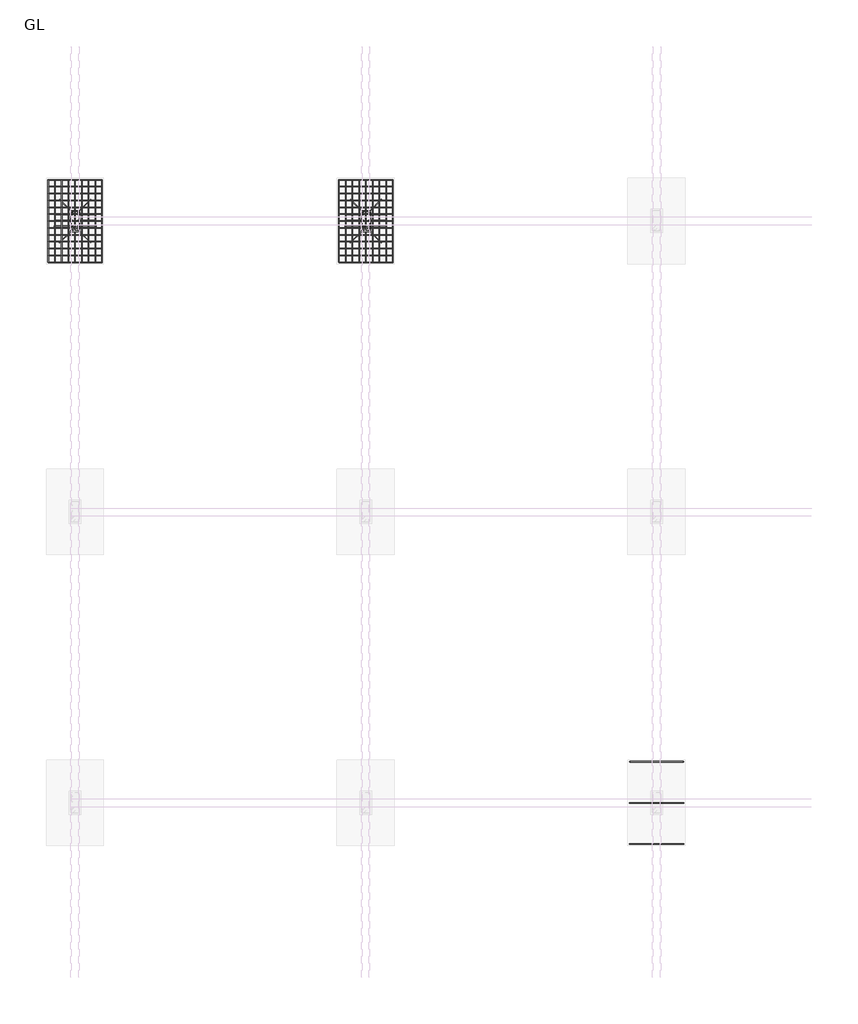
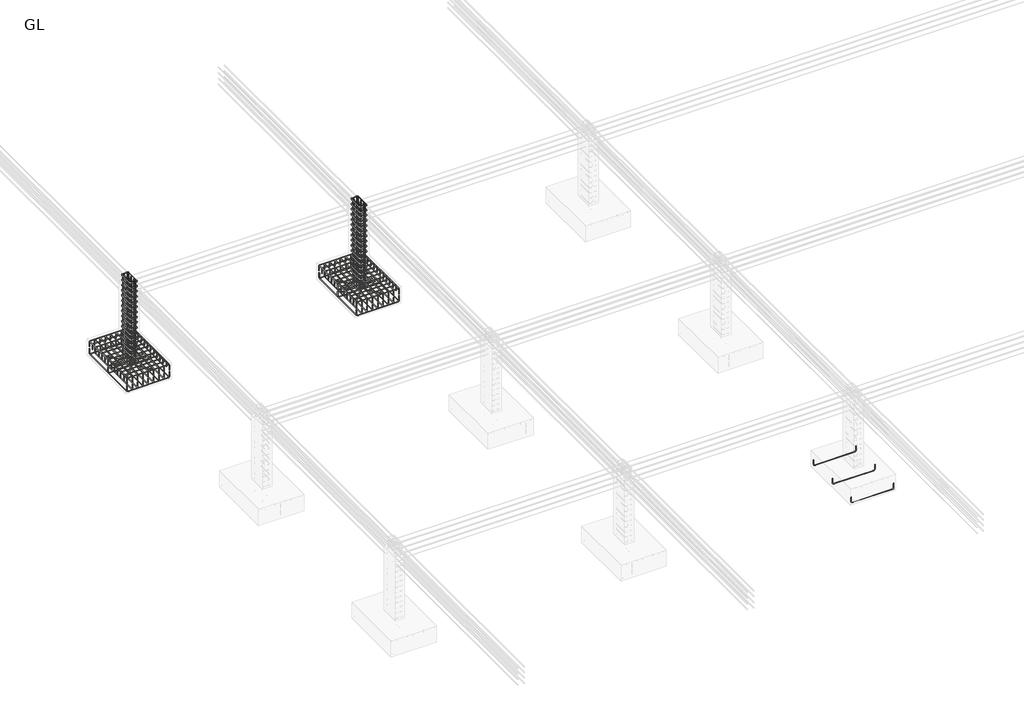
# One storey, part 6 of 16: 23 reinforcing bars.
"""IFC4 building model written with IfcOpenShell, lengths in millimetres."""

from ifc_helpers import new_model, si_unit, point, frame, origin, place, context, project, spatial, polyline, circle_curve, trimmed, segment, composite_curve, source, transform, mapped, element, save
from ifc_brep_helpers import swept_disk

model = new_model("IFC4")

# Units and contexts
model_context = context("Model", 3, world=origin())
ifc_project = project(units=[si_unit("LENGTHUNIT", "METRE", prefix="MILLI")], contexts=[model_context])

# Site, building, storey
site = spatial("IfcSite", under=ifc_project)
building = spatial("IfcBuilding", under=site)
storey = spatial("IfcBuildingStorey", under=building, Name="GL", Elevation=-1829.0)

# Reinforcing bars
placement = place(None, origin())
reinforcing_bar_shape = source(origin(), model_context, "Body", "SolidModel", [
    swept_disk(composite_curve([segment(polyline([(-16146.9544379, -1127.1167521, -2089.0), (-16146.9544379, -1127.1167521, -2213.0)]), True, "CONTINUOUS"), segment(trimmed(circle_curve(frame((-16176.9544379, -1127.1167521, -2213.0), z_axis=(0.0, 1.0, 0.0), x_axis=(30.0, 0.0, 0.0)), 30.0), [point((-16146.9544379, -1127.1167521, -2213.0))], [point((-16176.9544379, -1127.1167521, -2243.0))], True, "CARTESIAN"), True, "CONTINUOUS"), segment(polyline([(-16176.9544379, -1127.1167521, -2243.0), (-17244.9544379, -1127.1167521, -2243.0)]), True, "CONTINUOUS"), segment(trimmed(circle_curve(frame((-17244.9544379, -1127.1167521, -2213.0), z_axis=(0.0, 1.0, 0.0), x_axis=(0.0, 0.0, -30.0)), 30.0), [point((-17244.9544379, -1127.1167521, -2243.0))], [point((-17274.9544379, -1127.1167521, -2213.0))], True, "CARTESIAN"), True, "CONTINUOUS"), segment(polyline([(-17274.9544379, -1127.1167521, -2213.0), (-17274.9544379, -1127.1167521, -2089.0)]), True, "CONTINUOUS")], self_intersect=False), 6.0),
])
element("IfcReinforcingBar", 1, at=placement, inside=storey, context=model_context, shape_type="MappedRepresentation", body=[
    mapped(reinforcing_bar_shape, transform((0.0, 0.0, 0.0), x_axis=(1.0, 0.0, 0.0), y_axis=(0.0, 1.0, 0.0), z_axis=(0.0, 0.0, 1.0))),
    mapped(reinforcing_bar_shape, transform((0.0, -864.0, 0.0), x_axis=(1.0, 0.0, 0.0), y_axis=(0.0, 1.0, 0.0), z_axis=(0.0, 0.0, 1.0))),
    mapped(reinforcing_bar_shape, transform((0.0, -1728.0, 0.0), x_axis=(1.0, 0.0, 0.0), y_axis=(0.0, 1.0, 0.0), z_axis=(0.0, 0.0, 1.0))),
])
reinforcing_bar_2_shape = source(origin(), model_context, "Body", "SolidModel", [
    swept_disk(composite_curve([segment(polyline([(-17274.9544379, -1127.1167521, -2022.436678), (-17274.9544379, -1127.1167521, -1898.436678)]), True, "CONTINUOUS"), segment(trimmed(circle_curve(frame((-17244.9544379, -1127.1167521, -1898.436678), z_axis=(0.0, 1.0, 0.0), x_axis=(-30.0, 0.0, 0.0)), 30.0), [point((-17274.9544379, -1127.1167521, -1898.436678))], [point((-17244.9544379, -1127.1167521, -1868.436678))], True, "CARTESIAN"), True, "CONTINUOUS"), segment(polyline([(-17244.9544379, -1127.1167521, -1868.436678), (-16176.9544379, -1127.1167521, -1868.436678)]), True, "CONTINUOUS"), segment(trimmed(circle_curve(frame((-16176.9544379, -1127.1167521, -1898.436678), z_axis=(0.0, 1.0, 0.0), x_axis=(0.0, 0.0, 30.0)), 30.0), [point((-16176.9544379, -1127.1167521, -1868.436678))], [point((-16146.9544379, -1127.1167521, -1898.436678))], True, "CARTESIAN"), True, "CONTINUOUS"), segment(polyline([(-16146.9544379, -1127.1167521, -1898.436678), (-16146.9544379, -1127.1167521, -2022.436678)]), True, "CONTINUOUS")], self_intersect=False), 6.0),
])
element("IfcReinforcingBar", 2, at=placement, inside=storey, context=model_context, shape_type="MappedRepresentation", body=[
    mapped(reinforcing_bar_2_shape, transform((0.0, 0.0, 0.0), x_axis=(1.0, 0.0, 0.0), y_axis=(0.0, 1.0, 0.0), z_axis=(0.0, 0.0, 1.0))),
    mapped(reinforcing_bar_2_shape, transform((0.0, -144.0, 0.0), x_axis=(1.0, 0.0, 0.0), y_axis=(0.0, 1.0, 0.0), z_axis=(0.0, 0.0, 1.0))),
    mapped(reinforcing_bar_2_shape, transform((0.0, -288.0, 0.0), x_axis=(1.0, 0.0, 0.0), y_axis=(0.0, 1.0, 0.0), z_axis=(0.0, 0.0, 1.0))),
    mapped(reinforcing_bar_2_shape, transform((0.0, -432.0, 0.0), x_axis=(1.0, 0.0, 0.0), y_axis=(0.0, 1.0, 0.0), z_axis=(0.0, 0.0, 1.0))),
    mapped(reinforcing_bar_2_shape, transform((0.0, -576.0, 0.0), x_axis=(1.0, 0.0, 0.0), y_axis=(0.0, 1.0, 0.0), z_axis=(0.0, 0.0, 1.0))),
    mapped(reinforcing_bar_2_shape, transform((0.0, -720.0, 0.0), x_axis=(1.0, 0.0, 0.0), y_axis=(0.0, 1.0, 0.0), z_axis=(0.0, 0.0, 1.0))),
    mapped(reinforcing_bar_2_shape, transform((0.0, -864.0, 0.0), x_axis=(1.0, 0.0, 0.0), y_axis=(0.0, 1.0, 0.0), z_axis=(0.0, 0.0, 1.0))),
    mapped(reinforcing_bar_2_shape, transform((0.0, -1008.0, 0.0), x_axis=(1.0, 0.0, 0.0), y_axis=(0.0, 1.0, 0.0), z_axis=(0.0, 0.0, 1.0))),
    mapped(reinforcing_bar_2_shape, transform((0.0, -1152.0, 0.0), x_axis=(1.0, 0.0, 0.0), y_axis=(0.0, 1.0, 0.0), z_axis=(0.0, 0.0, 1.0))),
    mapped(reinforcing_bar_2_shape, transform((0.0, -1296.0, 0.0), x_axis=(1.0, 0.0, 0.0), y_axis=(0.0, 1.0, 0.0), z_axis=(0.0, 0.0, 1.0))),
    mapped(reinforcing_bar_2_shape, transform((0.0, -1440.0, 0.0), x_axis=(1.0, 0.0, 0.0), y_axis=(0.0, 1.0, 0.0), z_axis=(0.0, 0.0, 1.0))),
    mapped(reinforcing_bar_2_shape, transform((0.0, -1584.0, 0.0), x_axis=(1.0, 0.0, 0.0), y_axis=(0.0, 1.0, 0.0), z_axis=(0.0, 0.0, 1.0))),
    mapped(reinforcing_bar_2_shape, transform((0.0, -1728.0, 0.0), x_axis=(1.0, 0.0, 0.0), y_axis=(0.0, 1.0, 0.0), z_axis=(0.0, 0.0, 1.0))),
])
reinforcing_bar_3_shape = source(origin(), model_context, "Body", "SolidModel", [
    swept_disk(composite_curve([segment(polyline([(-17274.9544379, -2855.1167521, -2027.5081232), (-17274.9544379, -2855.1167521, -1903.5081232)]), True, "CONTINUOUS"), segment(trimmed(circle_curve(frame((-17274.9544379, -2825.1167521, -1903.5081232), z_axis=(-1.0, 0.0, 0.0), x_axis=(0.0, -30.0, 0.0)), 30.0), [point((-17274.9544379, -2855.1167521, -1903.5081232))], [point((-17274.9544379, -2825.1167521, -1873.5081232))], True, "CARTESIAN"), True, "CONTINUOUS"), segment(polyline([(-17274.9544379, -2825.1167521, -1873.5081232), (-17274.9544379, -1157.1167521, -1873.5081232)]), True, "CONTINUOUS"), segment(trimmed(circle_curve(frame((-17274.9544379, -1157.1167521, -1903.5081232), z_axis=(-1.0, 0.0, 0.0), x_axis=(0.0, 0.0, 30.0)), 30.0), [point((-17274.9544379, -1157.1167521, -1873.5081232))], [point((-17274.9544379, -1127.1167521, -1903.5081232))], True, "CARTESIAN"), True, "CONTINUOUS"), segment(polyline([(-17274.9544379, -1127.1167521, -1903.5081232), (-17274.9544379, -1127.1167521, -2027.5081232)]), True, "CONTINUOUS")], self_intersect=False), 6.0),
])
element("IfcReinforcingBar", 3, at=placement, inside=storey, context=model_context, shape_type="MappedRepresentation", body=[
    mapped(reinforcing_bar_3_shape, transform((0.0, 0.0, 0.0), x_axis=(1.0, 0.0, 0.0), y_axis=(0.0, 1.0, 0.0), z_axis=(0.0, 0.0, 1.0))),
    mapped(reinforcing_bar_3_shape, transform((141.0, 0.0, 0.0), x_axis=(1.0, 0.0, 0.0), y_axis=(0.0, 1.0, 0.0), z_axis=(0.0, 0.0, 1.0))),
    mapped(reinforcing_bar_3_shape, transform((282.0, 0.0, 0.0), x_axis=(1.0, 0.0, 0.0), y_axis=(0.0, 1.0, 0.0), z_axis=(0.0, 0.0, 1.0))),
    mapped(reinforcing_bar_3_shape, transform((423.0, 0.0, 0.0), x_axis=(1.0, 0.0, 0.0), y_axis=(0.0, 1.0, 0.0), z_axis=(0.0, 0.0, 1.0))),
    mapped(reinforcing_bar_3_shape, transform((564.0, 0.0, 0.0), x_axis=(1.0, 0.0, 0.0), y_axis=(0.0, 1.0, 0.0), z_axis=(0.0, 0.0, 1.0))),
    mapped(reinforcing_bar_3_shape, transform((705.0, 0.0, 0.0), x_axis=(1.0, 0.0, 0.0), y_axis=(0.0, 1.0, 0.0), z_axis=(0.0, 0.0, 1.0))),
    mapped(reinforcing_bar_3_shape, transform((846.0, 0.0, 0.0), x_axis=(1.0, 0.0, 0.0), y_axis=(0.0, 1.0, 0.0), z_axis=(0.0, 0.0, 1.0))),
    mapped(reinforcing_bar_3_shape, transform((987.0, 0.0, 0.0), x_axis=(1.0, 0.0, 0.0), y_axis=(0.0, 1.0, 0.0), z_axis=(0.0, 0.0, 1.0))),
    mapped(reinforcing_bar_3_shape, transform((1128.0, 0.0, 0.0), x_axis=(1.0, 0.0, 0.0), y_axis=(0.0, 1.0, 0.0), z_axis=(0.0, 0.0, 1.0))),
])
reinforcing_bar_4_shape = source(origin(), model_context, "Body", "SolidModel", [
    swept_disk(composite_curve([segment(polyline([(-16146.9544379, -2855.1167521, -2080.6239909), (-16146.9544379, -2855.1167521, -2204.6239909)]), True, "CONTINUOUS"), segment(trimmed(circle_curve(frame((-16146.9544379, -2825.1167521, -2204.6239909), z_axis=(1.0, 0.0, 0.0), x_axis=(0.0, -30.0, 0.0)), 30.0), [point((-16146.9544379, -2855.1167521, -2204.6239909))], [point((-16146.9544379, -2825.1167521, -2234.6239909))], True, "CARTESIAN"), True, "CONTINUOUS"), segment(polyline([(-16146.9544379, -2825.1167521, -2234.6239909), (-16146.9544379, -1170.1421892, -2234.6239909)]), True, "CONTINUOUS"), segment(trimmed(circle_curve(frame((-16146.9544379, -1170.1421892, -2204.6239909), z_axis=(1.0, 0.0, 0.0), x_axis=(0.0, 0.0, -30.0)), 30.0), [point((-16146.9544379, -1170.1421892, -2234.6239909))], [point((-16146.9544379, -1140.1421892, -2204.6239909))], True, "CARTESIAN"), True, "CONTINUOUS"), segment(polyline([(-16146.9544379, -1140.1421892, -2204.6239909), (-16146.9544379, -1140.1421892, -2080.6239909)]), True, "CONTINUOUS")], self_intersect=False), 6.0),
])
element("IfcReinforcingBar", 4, at=placement, inside=storey, context=model_context, shape_type="MappedRepresentation", body=[
    mapped(reinforcing_bar_4_shape, transform((0.0, 0.0, 0.0), x_axis=(1.0, 0.0, 0.0), y_axis=(0.0, 1.0, 0.0), z_axis=(0.0, 0.0, 1.0))),
    mapped(reinforcing_bar_4_shape, transform((-141.0, 0.0, 0.0), x_axis=(1.0, 0.0, 0.0), y_axis=(0.0, 1.0, 0.0), z_axis=(0.0, 0.0, 1.0))),
    mapped(reinforcing_bar_4_shape, transform((-282.0, 0.0, 0.0), x_axis=(1.0, 0.0, 0.0), y_axis=(0.0, 1.0, 0.0), z_axis=(0.0, 0.0, 1.0))),
    mapped(reinforcing_bar_4_shape, transform((-423.0, 0.0, 0.0), x_axis=(1.0, 0.0, 0.0), y_axis=(0.0, 1.0, 0.0), z_axis=(0.0, 0.0, 1.0))),
    mapped(reinforcing_bar_4_shape, transform((-564.0, 0.0, 0.0), x_axis=(1.0, 0.0, 0.0), y_axis=(0.0, 1.0, 0.0), z_axis=(0.0, 0.0, 1.0))),
    mapped(reinforcing_bar_4_shape, transform((-705.0, 0.0, 0.0), x_axis=(1.0, 0.0, 0.0), y_axis=(0.0, 1.0, 0.0), z_axis=(0.0, 0.0, 1.0))),
    mapped(reinforcing_bar_4_shape, transform((-846.0, 0.0, 0.0), x_axis=(1.0, 0.0, 0.0), y_axis=(0.0, 1.0, 0.0), z_axis=(0.0, 0.0, 1.0))),
    mapped(reinforcing_bar_4_shape, transform((-987.0, 0.0, 0.0), x_axis=(1.0, 0.0, 0.0), y_axis=(0.0, 1.0, 0.0), z_axis=(0.0, 0.0, 1.0))),
    mapped(reinforcing_bar_4_shape, transform((-1128.0, 0.0, 0.0), x_axis=(1.0, 0.0, 0.0), y_axis=(0.0, 1.0, 0.0), z_axis=(0.0, 0.0, 1.0))),
])
reinforcing_bar_5_shape = source(origin(), model_context, "Body", "SolidModel", [
    swept_disk(composite_curve([segment(polyline([(-22242.9544379, -1127.1167521, -2089.0), (-22242.9544379, -1127.1167521, -2213.0)]), True, "CONTINUOUS"), segment(trimmed(circle_curve(frame((-22272.9544379, -1127.1167521, -2213.0), z_axis=(0.0, 1.0, 0.0), x_axis=(30.0, 0.0, 0.0)), 30.0), [point((-22242.9544379, -1127.1167521, -2213.0))], [point((-22272.9544379, -1127.1167521, -2243.0))], True, "CARTESIAN"), True, "CONTINUOUS"), segment(polyline([(-22272.9544379, -1127.1167521, -2243.0), (-23340.9544379, -1127.1167521, -2243.0)]), True, "CONTINUOUS"), segment(trimmed(circle_curve(frame((-23340.9544379, -1127.1167521, -2213.0), z_axis=(0.0, 1.0, 0.0), x_axis=(0.0, 0.0, -30.0)), 30.0), [point((-23340.9544379, -1127.1167521, -2243.0))], [point((-23370.9544379, -1127.1167521, -2213.0))], True, "CARTESIAN"), True, "CONTINUOUS"), segment(polyline([(-23370.9544379, -1127.1167521, -2213.0), (-23370.9544379, -1127.1167521, -2089.0)]), True, "CONTINUOUS")], self_intersect=False), 6.0),
])
element("IfcReinforcingBar", 5, at=placement, inside=storey, context=model_context, shape_type="MappedRepresentation", body=[
    mapped(reinforcing_bar_5_shape, transform((0.0, 0.0, 0.0), x_axis=(1.0, 0.0, 0.0), y_axis=(0.0, 1.0, 0.0), z_axis=(0.0, 0.0, 1.0))),
    mapped(reinforcing_bar_5_shape, transform((0.0, -864.0, 0.0), x_axis=(1.0, 0.0, 0.0), y_axis=(0.0, 1.0, 0.0), z_axis=(0.0, 0.0, 1.0))),
    mapped(reinforcing_bar_5_shape, transform((0.0, -1728.0, 0.0), x_axis=(1.0, 0.0, 0.0), y_axis=(0.0, 1.0, 0.0), z_axis=(0.0, 0.0, 1.0))),
])
reinforcing_bar_6_shape = source(origin(), model_context, "Body", "SolidModel", [
    swept_disk(composite_curve([segment(polyline([(-23370.9544379, -1127.1167521, -2022.436678), (-23370.9544379, -1127.1167521, -1898.436678)]), True, "CONTINUOUS"), segment(trimmed(circle_curve(frame((-23340.9544379, -1127.1167521, -1898.436678), z_axis=(0.0, 1.0, 0.0), x_axis=(-30.0, 0.0, 0.0)), 30.0), [point((-23370.9544379, -1127.1167521, -1898.436678))], [point((-23340.9544379, -1127.1167521, -1868.436678))], True, "CARTESIAN"), True, "CONTINUOUS"), segment(polyline([(-23340.9544379, -1127.1167521, -1868.436678), (-22272.9544379, -1127.1167521, -1868.436678)]), True, "CONTINUOUS"), segment(trimmed(circle_curve(frame((-22272.9544379, -1127.1167521, -1898.436678), z_axis=(0.0, 1.0, 0.0), x_axis=(0.0, 0.0, 30.0)), 30.0), [point((-22272.9544379, -1127.1167521, -1868.436678))], [point((-22242.9544379, -1127.1167521, -1898.436678))], True, "CARTESIAN"), True, "CONTINUOUS"), segment(polyline([(-22242.9544379, -1127.1167521, -1898.436678), (-22242.9544379, -1127.1167521, -2022.436678)]), True, "CONTINUOUS")], self_intersect=False), 6.0),
])
element("IfcReinforcingBar", 6, at=placement, inside=storey, context=model_context, shape_type="MappedRepresentation", body=[
    mapped(reinforcing_bar_6_shape, transform((0.0, 0.0, 0.0), x_axis=(1.0, 0.0, 0.0), y_axis=(0.0, 1.0, 0.0), z_axis=(0.0, 0.0, 1.0))),
    mapped(reinforcing_bar_6_shape, transform((0.0, -144.0, 0.0), x_axis=(1.0, 0.0, 0.0), y_axis=(0.0, 1.0, 0.0), z_axis=(0.0, 0.0, 1.0))),
    mapped(reinforcing_bar_6_shape, transform((0.0, -288.0, 0.0), x_axis=(1.0, 0.0, 0.0), y_axis=(0.0, 1.0, 0.0), z_axis=(0.0, 0.0, 1.0))),
    mapped(reinforcing_bar_6_shape, transform((0.0, -432.0, 0.0), x_axis=(1.0, 0.0, 0.0), y_axis=(0.0, 1.0, 0.0), z_axis=(0.0, 0.0, 1.0))),
    mapped(reinforcing_bar_6_shape, transform((0.0, -576.0, 0.0), x_axis=(1.0, 0.0, 0.0), y_axis=(0.0, 1.0, 0.0), z_axis=(0.0, 0.0, 1.0))),
    mapped(reinforcing_bar_6_shape, transform((0.0, -720.0, 0.0), x_axis=(1.0, 0.0, 0.0), y_axis=(0.0, 1.0, 0.0), z_axis=(0.0, 0.0, 1.0))),
    mapped(reinforcing_bar_6_shape, transform((0.0, -864.0, 0.0), x_axis=(1.0, 0.0, 0.0), y_axis=(0.0, 1.0, 0.0), z_axis=(0.0, 0.0, 1.0))),
    mapped(reinforcing_bar_6_shape, transform((0.0, -1008.0, 0.0), x_axis=(1.0, 0.0, 0.0), y_axis=(0.0, 1.0, 0.0), z_axis=(0.0, 0.0, 1.0))),
    mapped(reinforcing_bar_6_shape, transform((0.0, -1152.0, 0.0), x_axis=(1.0, 0.0, 0.0), y_axis=(0.0, 1.0, 0.0), z_axis=(0.0, 0.0, 1.0))),
    mapped(reinforcing_bar_6_shape, transform((0.0, -1296.0, 0.0), x_axis=(1.0, 0.0, 0.0), y_axis=(0.0, 1.0, 0.0), z_axis=(0.0, 0.0, 1.0))),
    mapped(reinforcing_bar_6_shape, transform((0.0, -1440.0, 0.0), x_axis=(1.0, 0.0, 0.0), y_axis=(0.0, 1.0, 0.0), z_axis=(0.0, 0.0, 1.0))),
    mapped(reinforcing_bar_6_shape, transform((0.0, -1584.0, 0.0), x_axis=(1.0, 0.0, 0.0), y_axis=(0.0, 1.0, 0.0), z_axis=(0.0, 0.0, 1.0))),
    mapped(reinforcing_bar_6_shape, transform((0.0, -1728.0, 0.0), x_axis=(1.0, 0.0, 0.0), y_axis=(0.0, 1.0, 0.0), z_axis=(0.0, 0.0, 1.0))),
])
reinforcing_bar_7_shape = source(origin(), model_context, "Body", "SolidModel", [
    swept_disk(composite_curve([segment(polyline([(-23370.9544379, -2855.1167521, -2027.5081232), (-23370.9544379, -2855.1167521, -1903.5081232)]), True, "CONTINUOUS"), segment(trimmed(circle_curve(frame((-23370.9544379, -2825.1167521, -1903.5081232), z_axis=(-1.0, 0.0, 0.0), x_axis=(0.0, -30.0, 0.0)), 30.0), [point((-23370.9544379, -2855.1167521, -1903.5081232))], [point((-23370.9544379, -2825.1167521, -1873.5081232))], True, "CARTESIAN"), True, "CONTINUOUS"), segment(polyline([(-23370.9544379, -2825.1167521, -1873.5081232), (-23370.9544379, -1157.1167521, -1873.5081232)]), True, "CONTINUOUS"), segment(trimmed(circle_curve(frame((-23370.9544379, -1157.1167521, -1903.5081232), z_axis=(-1.0, 0.0, 0.0), x_axis=(0.0, 0.0, 30.0)), 30.0), [point((-23370.9544379, -1157.1167521, -1873.5081232))], [point((-23370.9544379, -1127.1167521, -1903.5081232))], True, "CARTESIAN"), True, "CONTINUOUS"), segment(polyline([(-23370.9544379, -1127.1167521, -1903.5081232), (-23370.9544379, -1127.1167521, -2027.5081232)]), True, "CONTINUOUS")], self_intersect=False), 6.0),
])
element("IfcReinforcingBar", 7, at=placement, inside=storey, context=model_context, shape_type="MappedRepresentation", body=[
    mapped(reinforcing_bar_7_shape, transform((0.0, 0.0, 0.0), x_axis=(1.0, 0.0, 0.0), y_axis=(0.0, 1.0, 0.0), z_axis=(0.0, 0.0, 1.0))),
    mapped(reinforcing_bar_7_shape, transform((141.0, 0.0, 0.0), x_axis=(1.0, 0.0, 0.0), y_axis=(0.0, 1.0, 0.0), z_axis=(0.0, 0.0, 1.0))),
    mapped(reinforcing_bar_7_shape, transform((282.0, 0.0, 0.0), x_axis=(1.0, 0.0, 0.0), y_axis=(0.0, 1.0, 0.0), z_axis=(0.0, 0.0, 1.0))),
    mapped(reinforcing_bar_7_shape, transform((423.0, 0.0, 0.0), x_axis=(1.0, 0.0, 0.0), y_axis=(0.0, 1.0, 0.0), z_axis=(0.0, 0.0, 1.0))),
    mapped(reinforcing_bar_7_shape, transform((564.0, 0.0, 0.0), x_axis=(1.0, 0.0, 0.0), y_axis=(0.0, 1.0, 0.0), z_axis=(0.0, 0.0, 1.0))),
    mapped(reinforcing_bar_7_shape, transform((705.0, 0.0, 0.0), x_axis=(1.0, 0.0, 0.0), y_axis=(0.0, 1.0, 0.0), z_axis=(0.0, 0.0, 1.0))),
    mapped(reinforcing_bar_7_shape, transform((846.0, 0.0, 0.0), x_axis=(1.0, 0.0, 0.0), y_axis=(0.0, 1.0, 0.0), z_axis=(0.0, 0.0, 1.0))),
    mapped(reinforcing_bar_7_shape, transform((987.0, 0.0, 0.0), x_axis=(1.0, 0.0, 0.0), y_axis=(0.0, 1.0, 0.0), z_axis=(0.0, 0.0, 1.0))),
    mapped(reinforcing_bar_7_shape, transform((1128.0, 0.0, 0.0), x_axis=(1.0, 0.0, 0.0), y_axis=(0.0, 1.0, 0.0), z_axis=(0.0, 0.0, 1.0))),
])
reinforcing_bar_8_shape = source(origin(), model_context, "Body", "SolidModel", [
    swept_disk(composite_curve([segment(polyline([(-22242.9544379, -2855.1167521, -2080.6239909), (-22242.9544379, -2855.1167521, -2204.6239909)]), True, "CONTINUOUS"), segment(trimmed(circle_curve(frame((-22242.9544379, -2825.1167521, -2204.6239909), z_axis=(1.0, 0.0, 0.0), x_axis=(0.0, -30.0, 0.0)), 30.0), [point((-22242.9544379, -2855.1167521, -2204.6239909))], [point((-22242.9544379, -2825.1167521, -2234.6239909))], True, "CARTESIAN"), True, "CONTINUOUS"), segment(polyline([(-22242.9544379, -2825.1167521, -2234.6239909), (-22242.9544379, -1170.1421892, -2234.6239909)]), True, "CONTINUOUS"), segment(trimmed(circle_curve(frame((-22242.9544379, -1170.1421892, -2204.6239909), z_axis=(1.0, 0.0, 0.0), x_axis=(0.0, 0.0, -30.0)), 30.0), [point((-22242.9544379, -1170.1421892, -2234.6239909))], [point((-22242.9544379, -1140.1421892, -2204.6239909))], True, "CARTESIAN"), True, "CONTINUOUS"), segment(polyline([(-22242.9544379, -1140.1421892, -2204.6239909), (-22242.9544379, -1140.1421892, -2080.6239909)]), True, "CONTINUOUS")], self_intersect=False), 6.0),
])
element("IfcReinforcingBar", 8, at=placement, inside=storey, context=model_context, shape_type="MappedRepresentation", body=[
    mapped(reinforcing_bar_8_shape, transform((0.0, 0.0, 0.0), x_axis=(1.0, 0.0, 0.0), y_axis=(0.0, 1.0, 0.0), z_axis=(0.0, 0.0, 1.0))),
    mapped(reinforcing_bar_8_shape, transform((-141.0, 0.0, 0.0), x_axis=(1.0, 0.0, 0.0), y_axis=(0.0, 1.0, 0.0), z_axis=(0.0, 0.0, 1.0))),
    mapped(reinforcing_bar_8_shape, transform((-282.0, 0.0, 0.0), x_axis=(1.0, 0.0, 0.0), y_axis=(0.0, 1.0, 0.0), z_axis=(0.0, 0.0, 1.0))),
    mapped(reinforcing_bar_8_shape, transform((-423.0, 0.0, 0.0), x_axis=(1.0, 0.0, 0.0), y_axis=(0.0, 1.0, 0.0), z_axis=(0.0, 0.0, 1.0))),
    mapped(reinforcing_bar_8_shape, transform((-564.0, 0.0, 0.0), x_axis=(1.0, 0.0, 0.0), y_axis=(0.0, 1.0, 0.0), z_axis=(0.0, 0.0, 1.0))),
    mapped(reinforcing_bar_8_shape, transform((-705.0, 0.0, 0.0), x_axis=(1.0, 0.0, 0.0), y_axis=(0.0, 1.0, 0.0), z_axis=(0.0, 0.0, 1.0))),
    mapped(reinforcing_bar_8_shape, transform((-846.0, 0.0, 0.0), x_axis=(1.0, 0.0, 0.0), y_axis=(0.0, 1.0, 0.0), z_axis=(0.0, 0.0, 1.0))),
    mapped(reinforcing_bar_8_shape, transform((-987.0, 0.0, 0.0), x_axis=(1.0, 0.0, 0.0), y_axis=(0.0, 1.0, 0.0), z_axis=(0.0, 0.0, 1.0))),
    mapped(reinforcing_bar_8_shape, transform((-1128.0, 0.0, 0.0), x_axis=(1.0, 0.0, 0.0), y_axis=(0.0, 1.0, 0.0), z_axis=(0.0, 0.0, 1.0))),
])
reinforcing_bar_9_shape = source(origin(), model_context, "Body", "SolidModel", [
    swept_disk(composite_curve([segment(polyline([(-10050.9544379, -13319.1167521, -2089.0), (-10050.9544379, -13319.1167521, -2213.0)]), True, "CONTINUOUS"), segment(trimmed(circle_curve(frame((-10080.9544379, -13319.1167521, -2213.0), z_axis=(0.0, 1.0, 0.0), x_axis=(30.0, 0.0, 0.0)), 30.0), [point((-10050.9544379, -13319.1167521, -2213.0))], [point((-10080.9544379, -13319.1167521, -2243.0))], True, "CARTESIAN"), True, "CONTINUOUS"), segment(polyline([(-10080.9544379, -13319.1167521, -2243.0), (-11148.9544379, -13319.1167521, -2243.0)]), True, "CONTINUOUS"), segment(trimmed(circle_curve(frame((-11148.9544379, -13319.1167521, -2213.0), z_axis=(0.0, 1.0, 0.0), x_axis=(0.0, 0.0, -30.0)), 30.0), [point((-11148.9544379, -13319.1167521, -2243.0))], [point((-11178.9544379, -13319.1167521, -2213.0))], True, "CARTESIAN"), True, "CONTINUOUS"), segment(polyline([(-11178.9544379, -13319.1167521, -2213.0), (-11178.9544379, -13319.1167521, -2089.0)]), True, "CONTINUOUS")], self_intersect=False), 6.0),
])
element("IfcReinforcingBar", 9, at=placement, inside=storey, context=model_context, shape_type="MappedRepresentation", body=[
    mapped(reinforcing_bar_9_shape, transform((0.0, 0.0, 0.0), x_axis=(1.0, 0.0, 0.0), y_axis=(0.0, 1.0, 0.0), z_axis=(0.0, 0.0, 1.0))),
    mapped(reinforcing_bar_9_shape, transform((0.0, -864.0, 0.0), x_axis=(1.0, 0.0, 0.0), y_axis=(0.0, 1.0, 0.0), z_axis=(0.0, 0.0, 1.0))),
    mapped(reinforcing_bar_9_shape, transform((0.0, -1728.0, 0.0), x_axis=(1.0, 0.0, 0.0), y_axis=(0.0, 1.0, 0.0), z_axis=(0.0, 0.0, 1.0))),
])
reinforcing_bar_10_shape = source(origin(), model_context, "Body", "SolidModel", [
    swept_disk(composite_curve([segment(polyline([(-22799.4864005, -2066.2223078, -1793.0), (-22887.1676414, -2153.9035486, -1793.0)]), True, "CONTINUOUS"), segment(trimmed(circle_curve(frame((-22865.9544379, -2175.1167521, -1793.0), z_axis=(0.0, 0.0, 1.0), x_axis=(-21.21320349999951, 21.213203500000418, 0.0)), 30.0), [point((-22887.1676414, -2153.9035486, -1793.0))], [point((-22865.9544379, -2205.1167521, -1793.0))], True, "CARTESIAN"), True, "CONTINUOUS"), segment(polyline([(-22865.9544379, -2205.1167521, -1793.0), (-22747.9544379, -2205.1167521, -1793.0)]), True, "CONTINUOUS"), segment(trimmed(circle_curve(frame((-22747.9544379, -2175.1167521, -1793.0), z_axis=(0.0, 0.0, 1.0), x_axis=(0.0, -30.0, 0.0)), 30.0), [point((-22747.9544379, -2205.1167521, -1793.0))], [point((-22717.9544379, -2175.1167521, -1793.0))], True, "CARTESIAN"), True, "CONTINUOUS"), segment(polyline([(-22717.9544379, -2175.1167521, -1793.0), (-22717.9544379, -1807.1167521, -1793.0)]), True, "CONTINUOUS"), segment(trimmed(circle_curve(frame((-22747.8864962, -1807.1167521, -1795.0178916), z_axis=(-0.06726305234213417, 0.0, 0.9977352764083365), x_axis=(29.93205830000079, 0.0, 2.0178915999999845)), 30.0), [point((-22717.9544379, -1807.1167521, -1793.0))], [point((-22747.8864962, -1777.1167521, -1795.0178916))], True, "CARTESIAN"), True, "CONTINUOUS"), segment(polyline([(-22747.8864962, -1777.1167521, -1795.0178916), (-22866.0223796, -1777.1167521, -1802.9821084)]), True, "CONTINUOUS"), segment(trimmed(circle_curve(frame((-22866.0223796, -1807.1167521, -1802.9821084), z_axis=(-0.06726305234213417, 0.0, 0.9977352764083365), x_axis=(0.0, 30.0, 0.0)), 30.0), [point((-22866.0223796, -1777.1167521, -1802.9821084))], [point((-22895.9544379, -1807.1167521, -1805.0))], True, "CARTESIAN"), True, "CONTINUOUS"), segment(polyline([(-22895.9544379, -1807.1167521, -1805.0), (-22895.9544379, -2175.1167521, -1805.0)]), True, "CONTINUOUS"), segment(trimmed(circle_curve(frame((-22865.9544379, -2175.1167521, -1805.0), z_axis=(0.0, 0.0, 1.0), x_axis=(-30.0, 0.0, 0.0)), 30.0), [point((-22895.9544379, -2175.1167521, -1805.0))], [point((-22844.7412345, -2196.3299555, -1805.0))], True, "CARTESIAN"), True, "CONTINUOUS"), segment(polyline([(-22844.7412345, -2196.3299555, -1805.0), (-22757.0599936, -2108.6487146, -1805.0)]), True, "CONTINUOUS")], self_intersect=False), 6.0),
])
element("IfcReinforcingBar", 10, at=placement, inside=storey, context=model_context, shape_type="MappedRepresentation", body=[
    mapped(reinforcing_bar_10_shape, transform((0.0, 0.0, 0.0), x_axis=(1.0, 0.0, 0.0), y_axis=(0.0, 1.0, 0.0), z_axis=(0.0, 0.0, 1.0))),
    mapped(reinforcing_bar_10_shape, transform((0.0, 0.0, 144.8571429), x_axis=(1.0, 0.0, 0.0), y_axis=(0.0, 1.0, 0.0), z_axis=(0.0, 0.0, 1.0))),
    mapped(reinforcing_bar_10_shape, transform((0.0, 0.0, 289.7142857), x_axis=(1.0, 0.0, 0.0), y_axis=(0.0, 1.0, 0.0), z_axis=(0.0, 0.0, 1.0))),
    mapped(reinforcing_bar_10_shape, transform((0.0, 0.0, 434.5714286), x_axis=(1.0, 0.0, 0.0), y_axis=(0.0, 1.0, 0.0), z_axis=(0.0, 0.0, 1.0))),
    mapped(reinforcing_bar_10_shape, transform((0.0, 0.0, 579.4285714), x_axis=(1.0, 0.0, 0.0), y_axis=(0.0, 1.0, 0.0), z_axis=(0.0, 0.0, 1.0))),
    mapped(reinforcing_bar_10_shape, transform((0.0, 0.0, 724.2857143), x_axis=(1.0, 0.0, 0.0), y_axis=(0.0, 1.0, 0.0), z_axis=(0.0, 0.0, 1.0))),
    mapped(reinforcing_bar_10_shape, transform((0.0, 0.0, 869.1428571), x_axis=(1.0, 0.0, 0.0), y_axis=(0.0, 1.0, 0.0), z_axis=(0.0, 0.0, 1.0))),
    mapped(reinforcing_bar_10_shape, transform((0.0, 0.0, 1014.0), x_axis=(1.0, 0.0, 0.0), y_axis=(0.0, 1.0, 0.0), z_axis=(0.0, 0.0, 1.0))),
    mapped(reinforcing_bar_10_shape, transform((0.0, 0.0, 1158.8571429), x_axis=(1.0, 0.0, 0.0), y_axis=(0.0, 1.0, 0.0), z_axis=(0.0, 0.0, 1.0))),
    mapped(reinforcing_bar_10_shape, transform((0.0, 0.0, 1303.7142857), x_axis=(1.0, 0.0, 0.0), y_axis=(0.0, 1.0, 0.0), z_axis=(0.0, 0.0, 1.0))),
    mapped(reinforcing_bar_10_shape, transform((0.0, 0.0, 1448.5714286), x_axis=(1.0, 0.0, 0.0), y_axis=(0.0, 1.0, 0.0), z_axis=(0.0, 0.0, 1.0))),
    mapped(reinforcing_bar_10_shape, transform((0.0, 0.0, 1593.4285714), x_axis=(1.0, 0.0, 0.0), y_axis=(0.0, 1.0, 0.0), z_axis=(0.0, 0.0, 1.0))),
    mapped(reinforcing_bar_10_shape, transform((0.0, 0.0, 1738.2857143), x_axis=(1.0, 0.0, 0.0), y_axis=(0.0, 1.0, 0.0), z_axis=(0.0, 0.0, 1.0))),
    mapped(reinforcing_bar_10_shape, transform((0.0, 0.0, 1883.1428571), x_axis=(1.0, 0.0, 0.0), y_axis=(0.0, 1.0, 0.0), z_axis=(0.0, 0.0, 1.0))),
    mapped(reinforcing_bar_10_shape, transform((0.0, 0.0, 2028.0), x_axis=(1.0, 0.0, 0.0), y_axis=(0.0, 1.0, 0.0), z_axis=(0.0, 0.0, 1.0))),
])
element("IfcReinforcingBar", 11, at=placement, inside=storey, context=model_context, shape_type="SolidModel", body=[
    swept_disk(composite_curve([segment(polyline([(-22864.0642232, -2176.0642439, 241.0), (-22864.0642232, -2176.0642439, -2129.0)]), True, "CONTINUOUS"), segment(trimmed(circle_curve(frame((-22885.2774266, -2197.2774473, -2129.0), z_axis=(-0.7071067811865187, 0.7071067811865764, 0.0), x_axis=(21.213203400002385, 21.21320340000011, 0.0)), 30.0), [point((-22864.0642232, -2176.0642439, -2129.0))], [point((-22885.2774266, -2197.2774473, -2159.0))], True, "CARTESIAN"), True, "CONTINUOUS"), segment(polyline([(-22885.2774266, -2197.2774473, -2159.0), (-23132.7648, -2444.7648207, -2159.0)]), True, "CONTINUOUS")], self_intersect=False), 6.0),
])
element("IfcReinforcingBar", 12, at=placement, inside=storey, context=model_context, shape_type="SolidModel", body=[
    swept_disk(composite_curve([segment(polyline([(-22864.0642232, -1806.1692603, 241.0), (-22864.0642232, -1806.1692603, -2129.0)]), True, "CONTINUOUS"), segment(trimmed(circle_curve(frame((-22885.2774266, -1784.9560568, -2129.0), z_axis=(0.7071067811865218, 0.7071067811865733, 0.0), x_axis=(21.213203400002385, -21.213203499999963, 0.0)), 30.0), [point((-22864.0642232, -1806.1692603, -2129.0))], [point((-22885.2774266, -1784.9560568, -2159.0))], True, "CARTESIAN"), True, "CONTINUOUS"), segment(polyline([(-22885.2774266, -1784.9560568, -2159.0), (-23132.7648, -1537.4686834, -2159.0)]), True, "CONTINUOUS")], self_intersect=False), 6.0),
])
element("IfcReinforcingBar", 13, at=placement, inside=storey, context=model_context, shape_type="SolidModel", body=[
    swept_disk(composite_curve([segment(polyline([(-22749.8446527, -2176.0642439, 241.0), (-22749.8446527, -2176.0642439, -2129.0)]), True, "CONTINUOUS"), segment(trimmed(circle_curve(frame((-22728.6314492, -2197.2774473, -2129.0), z_axis=(-0.7071067811865248, -0.7071067811865703, 0.0), x_axis=(-21.213203500003146, 21.21320340000011, 0.0)), 30.0), [point((-22749.8446527, -2176.0642439, -2129.0))], [point((-22728.6314492, -2197.2774473, -2159.0))], True, "CARTESIAN"), True, "CONTINUOUS"), segment(polyline([(-22728.6314492, -2197.2774473, -2159.0), (-22481.1440758, -2444.7648207, -2159.0)]), True, "CONTINUOUS")], self_intersect=False), 6.0),
])
element("IfcReinforcingBar", 14, at=placement, inside=storey, context=model_context, shape_type="SolidModel", body=[
    swept_disk(composite_curve([segment(polyline([(-22749.8446527, -1806.1692603, 241.0), (-22749.8446527, -1806.1692603, -2129.0)]), True, "CONTINUOUS"), segment(trimmed(circle_curve(frame((-22728.6314492, -1784.9560568, -2129.0), z_axis=(0.7071067811865157, -0.7071067811865794, 0.0), x_axis=(-21.213203500003146, -21.213203499999963, 0.0)), 30.0), [point((-22749.8446527, -1806.1692603, -2129.0))], [point((-22728.6314492, -1784.9560568, -2159.0))], True, "CARTESIAN"), True, "CONTINUOUS"), segment(polyline([(-22728.6314492, -1784.9560568, -2159.0), (-22481.1440758, -1537.4686834, -2159.0)]), True, "CONTINUOUS")], self_intersect=False), 6.0),
])
reinforcing_bar_11_shape = source(origin(), model_context, "Body", "SolidModel", [
    swept_disk(composite_curve([segment(polyline([(-22864.0642232, -2098.9117405, 241.0), (-22864.0642232, -2098.9117405, -2129.0)]), True, "CONTINUOUS"), segment(trimmed(circle_curve(frame((-22894.0642232, -2098.9117405, -2129.0), z_axis=(0.0, 1.0, 0.0), x_axis=(30.0, 0.0, 0.0)), 30.0), [point((-22864.0642232, -2098.9117405, -2129.0))], [point((-22894.0642232, -2098.9117405, -2159.0))], True, "CARTESIAN"), True, "CONTINUOUS"), segment(polyline([(-22894.0642232, -2098.9117405, -2159.0), (-23244.0642232, -2098.9117405, -2159.0)]), True, "CONTINUOUS")], self_intersect=False), 6.0),
])
element("IfcReinforcingBar", 15, at=placement, inside=storey, context=model_context, shape_type="MappedRepresentation", body=[
    mapped(reinforcing_bar_11_shape, transform((0.0, 0.0, 0.0), x_axis=(1.0, 0.0, 0.0), y_axis=(0.0, 1.0, 0.0), z_axis=(0.0, 0.0, 1.0))),
    mapped(reinforcing_bar_11_shape, transform((0.0, 123.5823926, 0.0), x_axis=(1.0, 0.0, 0.0), y_axis=(0.0, 1.0, 0.0), z_axis=(0.0, 0.0, 1.0))),
    mapped(reinforcing_bar_11_shape, transform((0.0, 247.1647853, 0.0), x_axis=(1.0, 0.0, 0.0), y_axis=(0.0, 1.0, 0.0), z_axis=(0.0, 0.0, 1.0))),
])
reinforcing_bar_12_shape = source(origin(), model_context, "Body", "SolidModel", [
    swept_disk(composite_curve([segment(polyline([(-22749.8446527, -2098.9117405, 241.0), (-22749.8446527, -2098.9117405, -2129.0)]), True, "CONTINUOUS"), segment(trimmed(circle_curve(frame((-22719.8446527, -2098.9117405, -2129.0), z_axis=(0.0, -1.0, 0.0), x_axis=(-30.0, 0.0, 0.0)), 30.0), [point((-22749.8446527, -2098.9117405, -2129.0))], [point((-22719.8446527, -2098.9117405, -2159.0))], True, "CARTESIAN"), True, "CONTINUOUS"), segment(polyline([(-22719.8446527, -2098.9117405, -2159.0), (-22369.8446527, -2098.9117405, -2159.0)]), True, "CONTINUOUS")], self_intersect=False), 6.0),
])
element("IfcReinforcingBar", 16, at=placement, inside=storey, context=model_context, shape_type="MappedRepresentation", body=[
    mapped(reinforcing_bar_12_shape, transform((0.0, 0.0, 0.0), x_axis=(1.0, 0.0, 0.0), y_axis=(0.0, 1.0, 0.0), z_axis=(0.0, 0.0, 1.0))),
    mapped(reinforcing_bar_12_shape, transform((0.0, 123.5823926, 0.0), x_axis=(1.0, 0.0, 0.0), y_axis=(0.0, 1.0, 0.0), z_axis=(0.0, 0.0, 1.0))),
    mapped(reinforcing_bar_12_shape, transform((0.0, 247.1647853, 0.0), x_axis=(1.0, 0.0, 0.0), y_axis=(0.0, 1.0, 0.0), z_axis=(0.0, 0.0, 1.0))),
])
reinforcing_bar_13_shape = source(origin(), model_context, "Body", "SolidModel", [
    swept_disk(composite_curve([segment(polyline([(-16703.4864005, -2066.2223078, -1793.0), (-16791.1676414, -2153.9035486, -1793.0)]), True, "CONTINUOUS"), segment(trimmed(circle_curve(frame((-16769.9544379, -2175.1167521, -1793.0), z_axis=(0.0, 0.0, 1.0), x_axis=(-21.21320349999951, 21.213203500000418, 0.0)), 30.0), [point((-16791.1676414, -2153.9035486, -1793.0))], [point((-16769.9544379, -2205.1167521, -1793.0))], True, "CARTESIAN"), True, "CONTINUOUS"), segment(polyline([(-16769.9544379, -2205.1167521, -1793.0), (-16651.9544379, -2205.1167521, -1793.0)]), True, "CONTINUOUS"), segment(trimmed(circle_curve(frame((-16651.9544379, -2175.1167521, -1793.0), z_axis=(0.0, 0.0, 1.0), x_axis=(0.0, -30.0, 0.0)), 30.0), [point((-16651.9544379, -2205.1167521, -1793.0))], [point((-16621.9544379, -2175.1167521, -1793.0))], True, "CARTESIAN"), True, "CONTINUOUS"), segment(polyline([(-16621.9544379, -2175.1167521, -1793.0), (-16621.9544379, -1807.1167521, -1793.0)]), True, "CONTINUOUS"), segment(trimmed(circle_curve(frame((-16651.8864962, -1807.1167521, -1795.0178916), z_axis=(-0.06726305234213417, 0.0, 0.9977352764083365), x_axis=(29.93205830000079, 0.0, 2.0178915999999845)), 30.0), [point((-16621.9544379, -1807.1167521, -1793.0))], [point((-16651.8864962, -1777.1167521, -1795.0178916))], True, "CARTESIAN"), True, "CONTINUOUS"), segment(polyline([(-16651.8864962, -1777.1167521, -1795.0178916), (-16770.0223796, -1777.1167521, -1802.9821084)]), True, "CONTINUOUS"), segment(trimmed(circle_curve(frame((-16770.0223796, -1807.1167521, -1802.9821084), z_axis=(-0.06726305234213417, 0.0, 0.9977352764083365), x_axis=(0.0, 30.0, 0.0)), 30.0), [point((-16770.0223796, -1777.1167521, -1802.9821084))], [point((-16799.9544379, -1807.1167521, -1805.0))], True, "CARTESIAN"), True, "CONTINUOUS"), segment(polyline([(-16799.9544379, -1807.1167521, -1805.0), (-16799.9544379, -2175.1167521, -1805.0)]), True, "CONTINUOUS"), segment(trimmed(circle_curve(frame((-16769.9544379, -2175.1167521, -1805.0), z_axis=(0.0, 0.0, 1.0), x_axis=(-30.0, 0.0, 0.0)), 30.0), [point((-16799.9544379, -2175.1167521, -1805.0))], [point((-16748.7412345, -2196.3299555, -1805.0))], True, "CARTESIAN"), True, "CONTINUOUS"), segment(polyline([(-16748.7412345, -2196.3299555, -1805.0), (-16661.0599936, -2108.6487146, -1805.0)]), True, "CONTINUOUS")], self_intersect=False), 6.0),
])
element("IfcReinforcingBar", 17, at=placement, inside=storey, context=model_context, shape_type="MappedRepresentation", body=[
    mapped(reinforcing_bar_13_shape, transform((0.0, 0.0, 0.0), x_axis=(1.0, 0.0, 0.0), y_axis=(0.0, 1.0, 0.0), z_axis=(0.0, 0.0, 1.0))),
    mapped(reinforcing_bar_13_shape, transform((0.0, 0.0, 144.8571429), x_axis=(1.0, 0.0, 0.0), y_axis=(0.0, 1.0, 0.0), z_axis=(0.0, 0.0, 1.0))),
    mapped(reinforcing_bar_13_shape, transform((0.0, 0.0, 289.7142857), x_axis=(1.0, 0.0, 0.0), y_axis=(0.0, 1.0, 0.0), z_axis=(0.0, 0.0, 1.0))),
    mapped(reinforcing_bar_13_shape, transform((0.0, 0.0, 434.5714286), x_axis=(1.0, 0.0, 0.0), y_axis=(0.0, 1.0, 0.0), z_axis=(0.0, 0.0, 1.0))),
    mapped(reinforcing_bar_13_shape, transform((0.0, 0.0, 579.4285714), x_axis=(1.0, 0.0, 0.0), y_axis=(0.0, 1.0, 0.0), z_axis=(0.0, 0.0, 1.0))),
    mapped(reinforcing_bar_13_shape, transform((0.0, 0.0, 724.2857143), x_axis=(1.0, 0.0, 0.0), y_axis=(0.0, 1.0, 0.0), z_axis=(0.0, 0.0, 1.0))),
    mapped(reinforcing_bar_13_shape, transform((0.0, 0.0, 869.1428571), x_axis=(1.0, 0.0, 0.0), y_axis=(0.0, 1.0, 0.0), z_axis=(0.0, 0.0, 1.0))),
    mapped(reinforcing_bar_13_shape, transform((0.0, 0.0, 1014.0), x_axis=(1.0, 0.0, 0.0), y_axis=(0.0, 1.0, 0.0), z_axis=(0.0, 0.0, 1.0))),
    mapped(reinforcing_bar_13_shape, transform((0.0, 0.0, 1158.8571429), x_axis=(1.0, 0.0, 0.0), y_axis=(0.0, 1.0, 0.0), z_axis=(0.0, 0.0, 1.0))),
    mapped(reinforcing_bar_13_shape, transform((0.0, 0.0, 1303.7142857), x_axis=(1.0, 0.0, 0.0), y_axis=(0.0, 1.0, 0.0), z_axis=(0.0, 0.0, 1.0))),
    mapped(reinforcing_bar_13_shape, transform((0.0, 0.0, 1448.5714286), x_axis=(1.0, 0.0, 0.0), y_axis=(0.0, 1.0, 0.0), z_axis=(0.0, 0.0, 1.0))),
    mapped(reinforcing_bar_13_shape, transform((0.0, 0.0, 1593.4285714), x_axis=(1.0, 0.0, 0.0), y_axis=(0.0, 1.0, 0.0), z_axis=(0.0, 0.0, 1.0))),
    mapped(reinforcing_bar_13_shape, transform((0.0, 0.0, 1738.2857143), x_axis=(1.0, 0.0, 0.0), y_axis=(0.0, 1.0, 0.0), z_axis=(0.0, 0.0, 1.0))),
    mapped(reinforcing_bar_13_shape, transform((0.0, 0.0, 1883.1428571), x_axis=(1.0, 0.0, 0.0), y_axis=(0.0, 1.0, 0.0), z_axis=(0.0, 0.0, 1.0))),
    mapped(reinforcing_bar_13_shape, transform((0.0, 0.0, 2028.0), x_axis=(1.0, 0.0, 0.0), y_axis=(0.0, 1.0, 0.0), z_axis=(0.0, 0.0, 1.0))),
])
element("IfcReinforcingBar", 18, at=placement, inside=storey, context=model_context, shape_type="SolidModel", body=[
    swept_disk(composite_curve([segment(polyline([(-16768.0642232, -2176.0642439, 241.0), (-16768.0642232, -2176.0642439, -2129.0)]), True, "CONTINUOUS"), segment(trimmed(circle_curve(frame((-16789.2774266, -2197.2774473, -2129.0), z_axis=(-0.7071067811865187, 0.7071067811865764, 0.0), x_axis=(21.213203400002385, 21.21320340000011, 0.0)), 30.0), [point((-16768.0642232, -2176.0642439, -2129.0))], [point((-16789.2774266, -2197.2774473, -2159.0))], True, "CARTESIAN"), True, "CONTINUOUS"), segment(polyline([(-16789.2774266, -2197.2774473, -2159.0), (-17036.7648, -2444.7648207, -2159.0)]), True, "CONTINUOUS")], self_intersect=False), 6.0),
])
element("IfcReinforcingBar", 19, at=placement, inside=storey, context=model_context, shape_type="SolidModel", body=[
    swept_disk(composite_curve([segment(polyline([(-16768.0642232, -1806.1692603, 241.0), (-16768.0642232, -1806.1692603, -2129.0)]), True, "CONTINUOUS"), segment(trimmed(circle_curve(frame((-16789.2774266, -1784.9560568, -2129.0), z_axis=(0.7071067811865218, 0.7071067811865733, 0.0), x_axis=(21.213203400002385, -21.213203499999963, 0.0)), 30.0), [point((-16768.0642232, -1806.1692603, -2129.0))], [point((-16789.2774266, -1784.9560568, -2159.0))], True, "CARTESIAN"), True, "CONTINUOUS"), segment(polyline([(-16789.2774266, -1784.9560568, -2159.0), (-17036.7648, -1537.4686834, -2159.0)]), True, "CONTINUOUS")], self_intersect=False), 6.0),
])
element("IfcReinforcingBar", 20, at=placement, inside=storey, context=model_context, shape_type="SolidModel", body=[
    swept_disk(composite_curve([segment(polyline([(-16653.8446527, -2176.0642439, 241.0), (-16653.8446527, -2176.0642439, -2129.0)]), True, "CONTINUOUS"), segment(trimmed(circle_curve(frame((-16632.6314492, -2197.2774473, -2129.0), z_axis=(-0.7071067811865248, -0.7071067811865703, 0.0), x_axis=(-21.213203500003146, 21.21320340000011, 0.0)), 30.0), [point((-16653.8446527, -2176.0642439, -2129.0))], [point((-16632.6314492, -2197.2774473, -2159.0))], True, "CARTESIAN"), True, "CONTINUOUS"), segment(polyline([(-16632.6314492, -2197.2774473, -2159.0), (-16385.1440758, -2444.7648207, -2159.0)]), True, "CONTINUOUS")], self_intersect=False), 6.0),
])
element("IfcReinforcingBar", 21, at=placement, inside=storey, context=model_context, shape_type="SolidModel", body=[
    swept_disk(composite_curve([segment(polyline([(-16653.8446527, -1806.1692603, 241.0), (-16653.8446527, -1806.1692603, -2129.0)]), True, "CONTINUOUS"), segment(trimmed(circle_curve(frame((-16632.6314492, -1784.9560568, -2129.0), z_axis=(0.7071067811865157, -0.7071067811865794, 0.0), x_axis=(-21.213203500003146, -21.213203499999963, 0.0)), 30.0), [point((-16653.8446527, -1806.1692603, -2129.0))], [point((-16632.6314492, -1784.9560568, -2159.0))], True, "CARTESIAN"), True, "CONTINUOUS"), segment(polyline([(-16632.6314492, -1784.9560568, -2159.0), (-16385.1440758, -1537.4686834, -2159.0)]), True, "CONTINUOUS")], self_intersect=False), 6.0),
])
reinforcing_bar_14_shape = source(origin(), model_context, "Body", "SolidModel", [
    swept_disk(composite_curve([segment(polyline([(-16768.0642232, -2098.9117405, 241.0), (-16768.0642232, -2098.9117405, -2129.0)]), True, "CONTINUOUS"), segment(trimmed(circle_curve(frame((-16798.0642232, -2098.9117405, -2129.0), z_axis=(0.0, 1.0, 0.0), x_axis=(30.0, 0.0, 0.0)), 30.0), [point((-16768.0642232, -2098.9117405, -2129.0))], [point((-16798.0642232, -2098.9117405, -2159.0))], True, "CARTESIAN"), True, "CONTINUOUS"), segment(polyline([(-16798.0642232, -2098.9117405, -2159.0), (-17148.0642232, -2098.9117405, -2159.0)]), True, "CONTINUOUS")], self_intersect=False), 6.0),
])
element("IfcReinforcingBar", 22, at=placement, inside=storey, context=model_context, shape_type="MappedRepresentation", body=[
    mapped(reinforcing_bar_14_shape, transform((0.0, 0.0, 0.0), x_axis=(1.0, 0.0, 0.0), y_axis=(0.0, 1.0, 0.0), z_axis=(0.0, 0.0, 1.0))),
    mapped(reinforcing_bar_14_shape, transform((0.0, 123.5823926, 0.0), x_axis=(1.0, 0.0, 0.0), y_axis=(0.0, 1.0, 0.0), z_axis=(0.0, 0.0, 1.0))),
    mapped(reinforcing_bar_14_shape, transform((0.0, 247.1647853, 0.0), x_axis=(1.0, 0.0, 0.0), y_axis=(0.0, 1.0, 0.0), z_axis=(0.0, 0.0, 1.0))),
])
reinforcing_bar_15_shape = source(origin(), model_context, "Body", "SolidModel", [
    swept_disk(composite_curve([segment(polyline([(-16653.8446527, -2098.9117405, 241.0), (-16653.8446527, -2098.9117405, -2129.0)]), True, "CONTINUOUS"), segment(trimmed(circle_curve(frame((-16623.8446527, -2098.9117405, -2129.0), z_axis=(0.0, -1.0, 0.0), x_axis=(-30.0, 0.0, 0.0)), 30.0), [point((-16653.8446527, -2098.9117405, -2129.0))], [point((-16623.8446527, -2098.9117405, -2159.0))], True, "CARTESIAN"), True, "CONTINUOUS"), segment(polyline([(-16623.8446527, -2098.9117405, -2159.0), (-16273.8446527, -2098.9117405, -2159.0)]), True, "CONTINUOUS")], self_intersect=False), 6.0),
])
element("IfcReinforcingBar", 23, at=placement, inside=storey, context=model_context, shape_type="MappedRepresentation", body=[
    mapped(reinforcing_bar_15_shape, transform((0.0, 0.0, 0.0), x_axis=(1.0, 0.0, 0.0), y_axis=(0.0, 1.0, 0.0), z_axis=(0.0, 0.0, 1.0))),
    mapped(reinforcing_bar_15_shape, transform((0.0, 123.5823926, 0.0), x_axis=(1.0, 0.0, 0.0), y_axis=(0.0, 1.0, 0.0), z_axis=(0.0, 0.0, 1.0))),
    mapped(reinforcing_bar_15_shape, transform((0.0, 247.1647853, 0.0), x_axis=(1.0, 0.0, 0.0), y_axis=(0.0, 1.0, 0.0), z_axis=(0.0, 0.0, 1.0))),
])

save(model, "model.ifc")

# Revit data of these elements
# Elements 1, 2, 3, 4, 5, 6, 7, 8, 9, 10, 11, 12, 13, 14, 15, 16, 17, 18, 19, 20, 21, 22, 23 (IfcReinforcingBar)
#   Phase Created = New Construction
